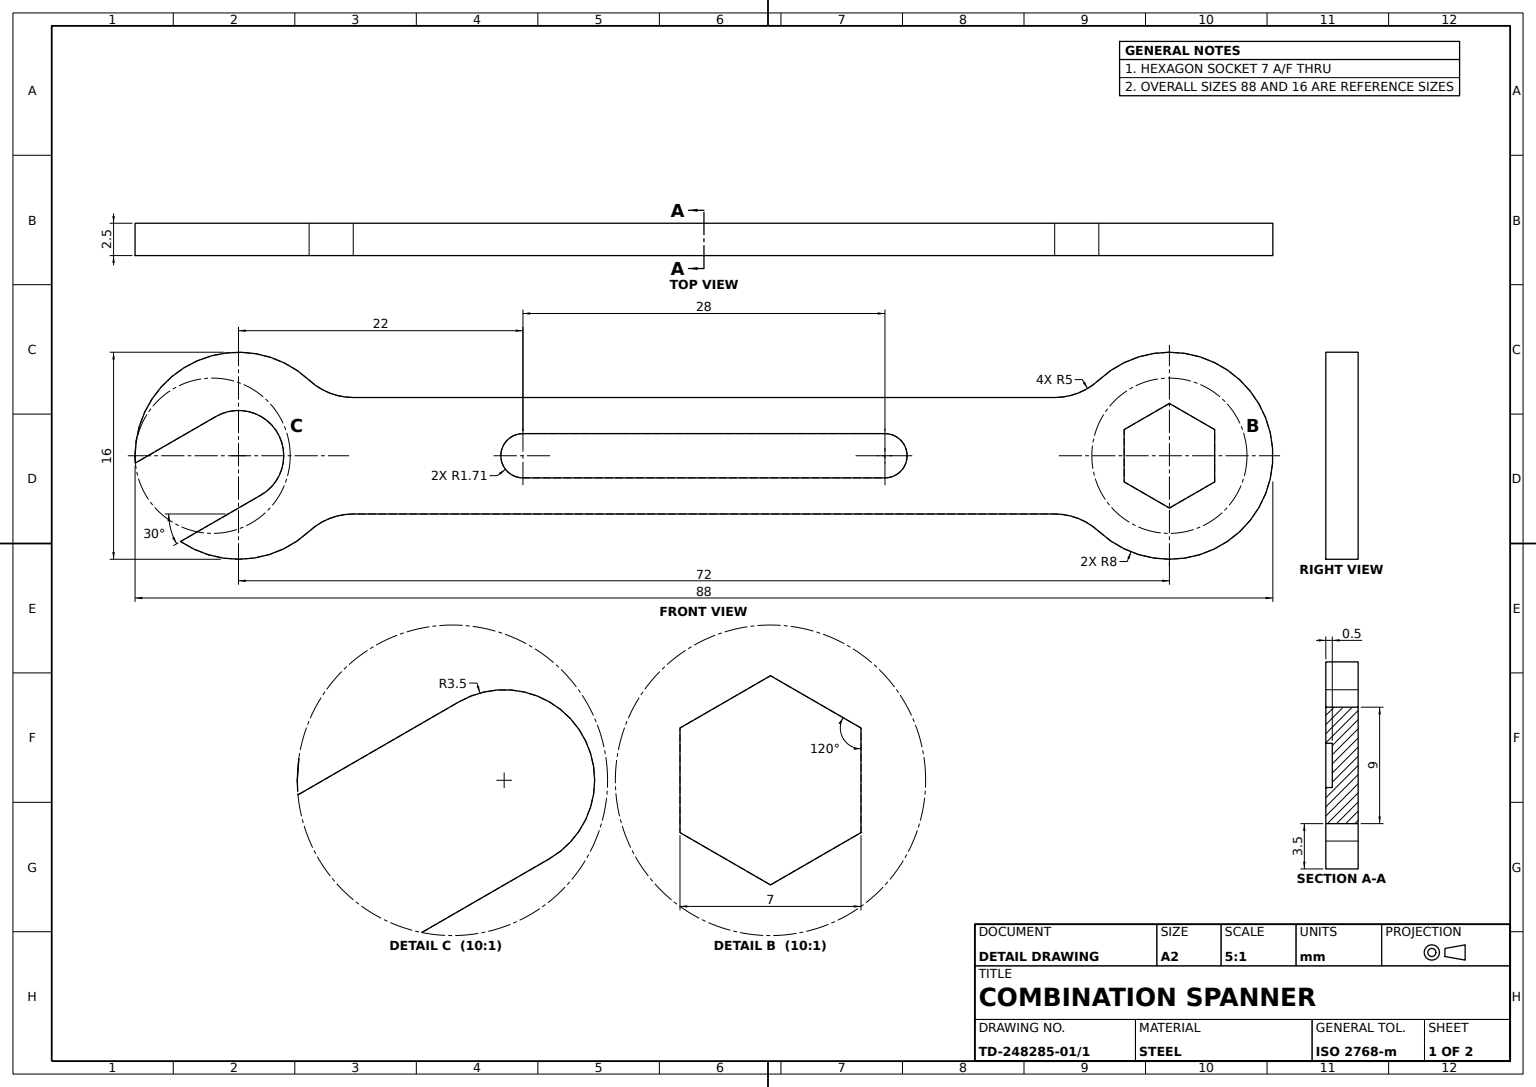
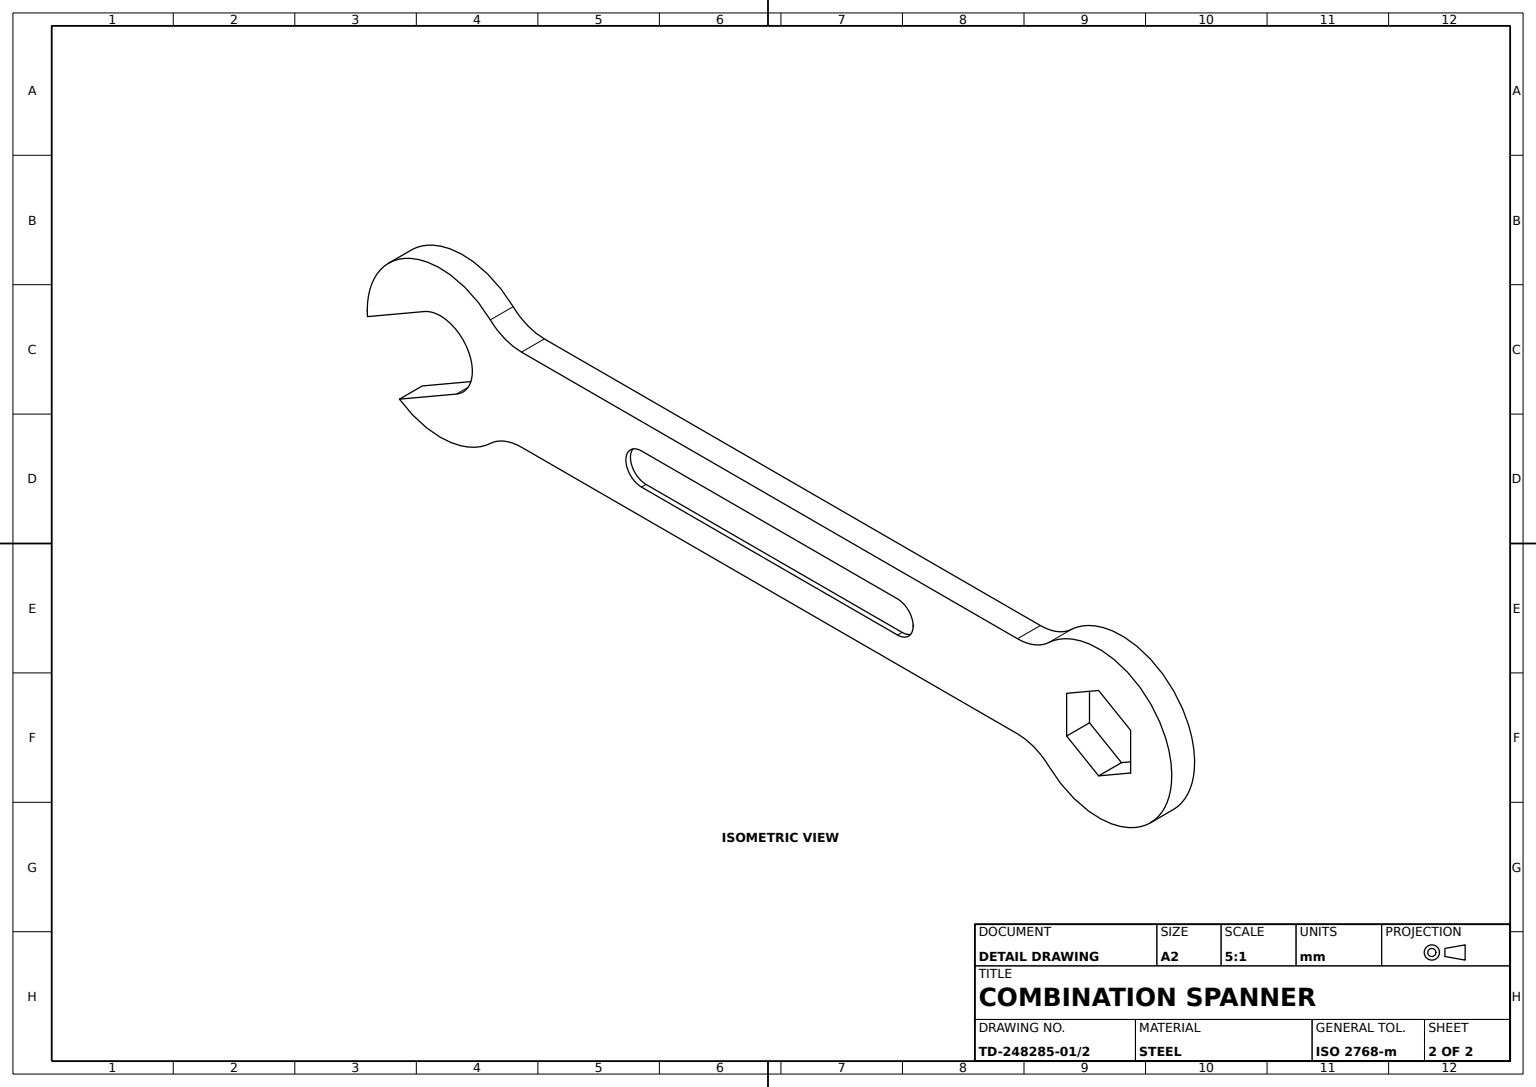
SolidWorks part; units mm, degrees
material "Plain Carbon Steel"
ref_plane "Front Plane" through (0, 0, 0) normal (0, 0, 1) x (1, 0, 0)
ref_plane "Top Plane" through (0, 0, 0) normal (0, 1, 0) x (1, 0, 0)
ref_plane "Right Plane" through (0, 0, 0) normal (1, 0, 0) x (0, 0, -1)
sketch "Spanner Outline Sketch" plane through (0, 0, 0) normal (0, 0, 1) x (1, 0, 0)
  line L0 (0, 0) -> (72, 0) construction
  line L1 (8.8741, -4.5) -> (63.1259, -4.5)
  line L2 (8.8741, 4.5) -> (63.1259, 4.5)
  line L3 (0, 0) -> (-12.5754, 0) construction
  line L4 (0, 4.5) -> (72, 4.5) construction
  line L5 (0, -4.5) -> (72, -4.5) construction
  line L7 (-1.75, 3.0311) -> (-7.98, -0.5658)
  line L8 (1.75, -3.0311) -> (-4.48, -6.628)
  line L9 (75.5, -2.0207) -> (75.5, 2.0207)
  line L10 (75.5, 2.0207) -> (72, 4.0415)
  line L11 (72, 4.0415) -> (68.5, 2.0207)
  line L12 (68.5, 2.0207) -> (68.5, -2.0207)
  line L13 (68.5, -2.0207) -> (72, -4.0415)
  line L14 (72, -4.0415) -> (75.5, -2.0207)
  arc A0 (1.75, -3.0311) -> (-1.75, 3.0311) centre (0, 0) ccw
  arc A1 (5.461, 5.8462) -> (-7.98, -0.5658) centre (0, 0) ccw
  arc A4 (5.461, 5.8462) -> (8.8741, 4.5) centre (8.8741, 9.5) ccw
  arc A5 (8.8741, -4.5) -> (5.461, -5.8462) centre (8.8741, -9.5) ccw
  arc A6 (-4.48, -6.628) -> (5.461, -5.8462) centre (0, 0) ccw
  circle A7 centre (72, 0) radius 3.5 construction
  arc A8 (63.1259, 4.5) -> (66.539, 5.8462) centre (63.1259, 9.5) ccw
  arc A9 (66.539, -5.8462) -> (63.1259, -4.5) centre (63.1259, -9.5) ccw
  arc A10 (66.539, -5.8462) -> (66.539, 5.8462) centre (72, 0) ccw
  point P21 (-15.8138, -5.0886)
  point P23 (-12.3138, -11.1508)
  dimension "D1" = 7
  dimension "D2" = 16
  dimension "D3" = 63.1259
  dimension "D4" = 7
  dimension "D8" = 5
  dimension "D9" = 5
  dimension "D14" = 5
  dimension "D15" = 66.539
  dimension "D16" = 5
  dimension "D5" = 4.5
  dimension "D7" = 72
  dimension "D10" = 7.98
  dimension "D11" = 6.628
  dimension "D12" = 1.75
  dimension "D13" = 3.0311
  dimension "D17" = 66.539
  dimension "D6" = 4.5
extrude "Spanner Body 2.5mm" add sketch "Spanner Outline Sketch" along normal blind 2.5
sketch "Handle Slot Sketch" plane through (0, 0, 2.5) normal (0, 0, 1) x (1, 0, 0)
  line L0 (22, 0) -> (50, 0) construction
  line L1 (22, 1.7111) -> (50, 1.7111)
  line L2 (22, -1.7111) -> (50, -1.7111)
  arc A0 (22, 1.7111) -> (22, -1.7111) centre (22, 0) ccw
  arc A1 (50, -1.7111) -> (50, 1.7111) centre (50, 0) ccw
  point P3 (36, 0)
  dimension "D3" = 1.7111
  dimension "D1" = 22
  dimension "D2" = 28
extrude "Handle Slot Recess 0.5mm" cut sketch "Handle Slot Sketch" against normal blind 0.5
